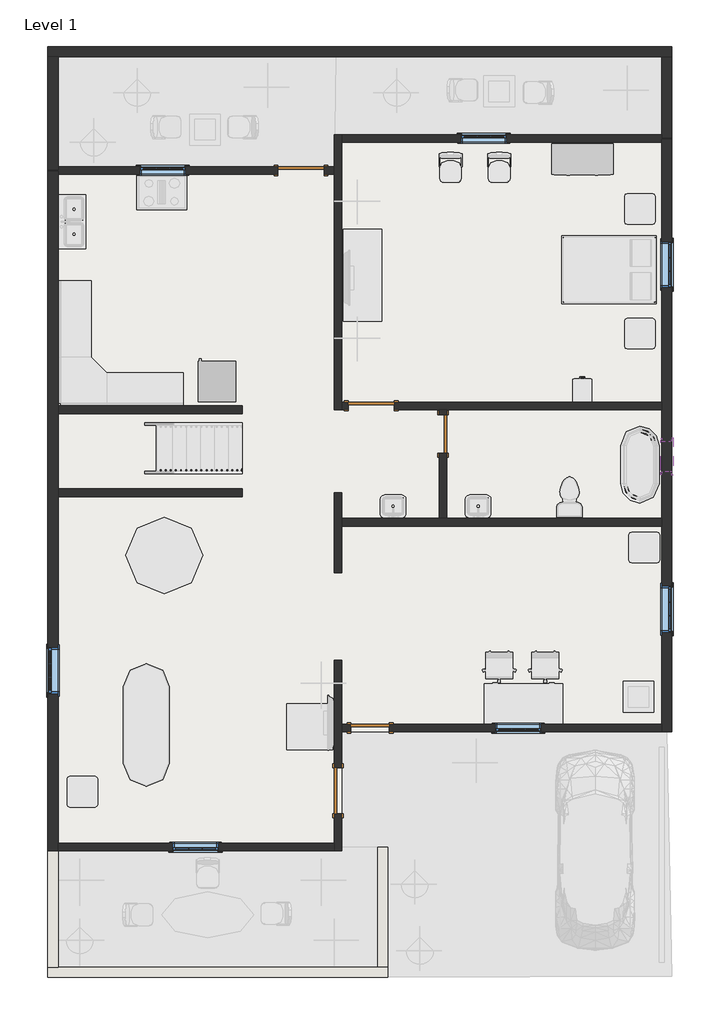
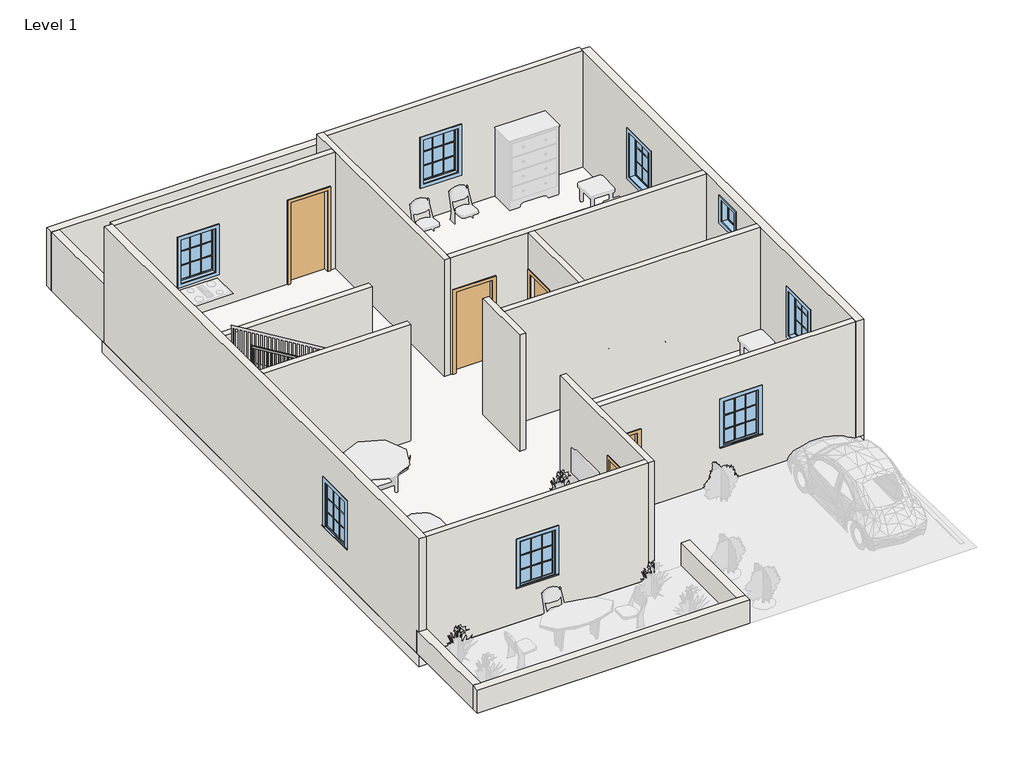
# One storey, part 1 of 2: 20 walls, 8 windows, 5 doors, 1 railing, 1 slab.
"""IFC4 building model written with IfcOpenShell, lengths in millimetres."""

from ifc_helpers import new_model, si_unit, frame, origin, origin_with_axes, place, context, project, spatial, polyline, outline, extrude, faceted_brep, transform, mapped, element, save
from components import door_255cab33, door_16372e1c, door_686f89d2, window_5c190c7e, window_29c06734, window_e41d21a6

model = new_model("IFC4")

# Units and contexts
model_context = context("Model", 3, world=origin())
ifc_project = project(units=[si_unit("LENGTHUNIT", "METRE", prefix="MILLI")], contexts=[model_context])

# Site, building, storey
site = spatial("IfcSite", under=ifc_project)
building = spatial("IfcBuilding", under=site)
storey = spatial("IfcBuildingStorey", under=building, Name="Level 1", Elevation=0.0)

# Doors
placement = place(None, origin())
door_shape = door_255cab33(model_context)
element("IfcDoor", 1, ObjectType="Single-Flush : 30\" x 80\"", at=placement, inside=storey, context=model_context, shape_type="MappedRepresentation", body=[
    mapped(door_shape, transform((1593.6745853, 5123.5742707, 0.0), x_axis=(0.0, 1.0, 0.0), y_axis=(-1.0, 0.0, 0.0), z_axis=(0.0, 0.0, 1.0))),
])
element("IfcDoor", 2, ObjectType="Single-Flush : 30\" x 80\"", at=placement, inside=storey, context=model_context, shape_type="MappedRepresentation", body=[
    mapped(door_shape, transform((145.8745853, -718.4257293, 0.0), x_axis=(-1.0, 0.0, 0.0), y_axis=(0.0, -1.0, 0.0), z_axis=(0.0, 0.0, 1.0))),
])
door_2_shape = door_16372e1c(model_context)
element("IfcDoor", 3, ObjectType="Single-Flush : 36\" x 84\"", at=placement, inside=storey, context=model_context, shape_type="MappedRepresentation", body=[
    mapped(door_2_shape, transform((-1225.7254147, 10355.9742707, 0.0), x_axis=(1.0, 0.0, 0.0), y_axis=(0.0, 1.0, 0.0), z_axis=(0.0, 0.0, 1.0))),
])
element("IfcDoor", 4, ObjectType="Single-Flush : 36\" x 84\"", at=placement, inside=storey, context=model_context, shape_type="MappedRepresentation", body=[
    mapped(door_2_shape, transform((-489.1254147, -1963.0257293, 0.0), x_axis=(0.0, 1.0, 0.0), y_axis=(-1.0, 0.0, 0.0), z_axis=(0.0, 0.0, 1.0))),
])
door_3_shape = door_686f89d2(model_context)
element("IfcDoor", 5, ObjectType="Single-Flush : 36\" x 84\"", at=placement, inside=storey, context=model_context, shape_type="MappedRepresentation", body=[
    mapped(door_3_shape, transform((171.2745853, 5682.3742707, 0.0), x_axis=(-1.0, 0.0, 0.0), y_axis=(0.0, -1.0, 0.0), z_axis=(0.0, 0.0, 1.0))),
])

# Railing
element("IfcRailing", 6, ObjectType="Handrail - Rectangular", at=placement, inside=storey, context=model_context, shape_type="SweptSolid", body=[
    extrude(outline(polyline([(1193.6652064, -2390.4214984), (1253.0666667, -2390.4214984), (3454.4, -6022.6214984), (3394.9985397, -6022.6214984), (1193.6652064, -2390.4214984)])), frame((0.0, 4382.4166905, 0.0), z_axis=(0.0, 1.0, 0.0), x_axis=(0.0, 0.0, 1.0)), (0.0, 0.0, 1.0), 50.8),
    extrude(outline(polyline([(3354.5894488, -5955.9464984), (2370.6666667, -5955.9464984), (2370.6666667, -5936.8964984), (3343.0439943, -5936.8964984), (3354.5894488, -5955.9464984)])), frame((0.0, 4398.2916905, 0.0), z_axis=(0.0, 1.0, 0.0), x_axis=(0.0, 0.0, 1.0)), (0.0, 0.0, 1.0), 19.05),
    extrude(outline(polyline([(3293.0136913, -5854.3464984), (2370.6666667, -5854.3464984), (2370.6666667, -5835.2964984), (3281.4682367, -5835.2964984), (3293.0136913, -5854.3464984)])), frame((0.0, 4398.2916905, 0.0), z_axis=(0.0, 1.0, 0.0), x_axis=(0.0, 0.0, 1.0)), (0.0, 0.0, 1.0), 19.05),
    extrude(outline(polyline([(3231.4379337, -5752.7464984), (2370.6666667, -5752.7464984), (2370.6666667, -5733.6964984), (3219.8924791, -5733.6964984), (3231.4379337, -5752.7464984)])), frame((0.0, 4398.2916905, 0.0), z_axis=(0.0, 1.0, 0.0), x_axis=(0.0, 0.0, 1.0)), (0.0, 0.0, 1.0), 19.05),
    extrude(outline(polyline([(3169.8621761, -5651.1464984), (2201.3333333, -5651.1464984), (2201.3333333, -5632.0964984), (3158.3167216, -5632.0964984), (3169.8621761, -5651.1464984)])), frame((0.0, 4398.2916905, 0.0), z_axis=(0.0, 1.0, 0.0), x_axis=(0.0, 0.0, 1.0)), (0.0, 0.0, 1.0), 19.05),
    extrude(outline(polyline([(3108.2864185, -5549.5464984), (2201.3333333, -5549.5464984), (2201.3333333, -5530.4964984), (3096.740964, -5530.4964984), (3108.2864185, -5549.5464984)])), frame((0.0, 4398.2916905, 0.0), z_axis=(0.0, 1.0, 0.0), x_axis=(0.0, 0.0, 1.0)), (0.0, 0.0, 1.0), 19.05),
    extrude(outline(polyline([(3046.710661, -5447.9464984), (2032.0, -5447.9464984), (2032.0, -5428.8964984), (3035.1652064, -5428.8964984), (3046.710661, -5447.9464984)])), frame((0.0, 4398.2916905, 0.0), z_axis=(0.0, 1.0, 0.0), x_axis=(0.0, 0.0, 1.0)), (0.0, 0.0, 1.0), 19.05),
    extrude(outline(polyline([(2985.1349034, -5346.3464984), (2032.0, -5346.3464984), (2032.0, -5327.2964984), (2973.5894488, -5327.2964984), (2985.1349034, -5346.3464984)])), frame((0.0, 4398.2916905, 0.0), z_axis=(0.0, 1.0, 0.0), x_axis=(0.0, 0.0, 1.0)), (0.0, 0.0, 1.0), 19.05),
    extrude(outline(polyline([(2923.5591458, -5244.7464984), (2032.0, -5244.7464984), (2032.0, -5225.6964984), (2912.0136913, -5225.6964984), (2923.5591458, -5244.7464984)])), frame((0.0, 4398.2916905, 0.0), z_axis=(0.0, 1.0, 0.0), x_axis=(0.0, 0.0, 1.0)), (0.0, 0.0, 1.0), 19.05),
    extrude(outline(polyline([(2861.9833882, -5143.1464984), (1862.6666667, -5143.1464984), (1862.6666667, -5124.0964984), (2850.4379337, -5124.0964984), (2861.9833882, -5143.1464984)])), frame((0.0, 4398.2916905, 0.0), z_axis=(0.0, 1.0, 0.0), x_axis=(0.0, 0.0, 1.0)), (0.0, 0.0, 1.0), 19.05),
    extrude(outline(polyline([(2800.4076307, -5041.5464984), (1862.6666667, -5041.5464984), (1862.6666667, -5022.4964984), (2788.8621761, -5022.4964984), (2800.4076307, -5041.5464984)])), frame((0.0, 4398.2916905, 0.0), z_axis=(0.0, 1.0, 0.0), x_axis=(0.0, 0.0, 1.0)), (0.0, 0.0, 1.0), 19.05),
    extrude(outline(polyline([(2738.8318731, -4939.9464984), (1862.6666667, -4939.9464984), (1862.6666667, -4920.8964984), (2727.2864185, -4920.8964984), (2738.8318731, -4939.9464984)])), frame((0.0, 4398.2916905, 0.0), z_axis=(0.0, 1.0, 0.0), x_axis=(0.0, 0.0, 1.0)), (0.0, 0.0, 1.0), 19.05),
    extrude(outline(polyline([(2677.2561155, -4838.3464984), (1693.3333333, -4838.3464984), (1693.3333333, -4819.2964984), (2665.710661, -4819.2964984), (2677.2561155, -4838.3464984)])), frame((0.0, 4398.2916905, 0.0), z_axis=(0.0, 1.0, 0.0), x_axis=(0.0, 0.0, 1.0)), (0.0, 0.0, 1.0), 19.05),
    extrude(outline(polyline([(2615.6803579, -4736.7464984), (1693.3333333, -4736.7464984), (1693.3333333, -4717.6964984), (2604.1349034, -4717.6964984), (2615.6803579, -4736.7464984)])), frame((0.0, 4398.2916905, 0.0), z_axis=(0.0, 1.0, 0.0), x_axis=(0.0, 0.0, 1.0)), (0.0, 0.0, 1.0), 19.05),
    extrude(outline(polyline([(2554.1046004, -4635.1464984), (1693.3333333, -4635.1464984), (1693.3333333, -4616.0964984), (2542.5591458, -4616.0964984), (2554.1046004, -4635.1464984)])), frame((0.0, 4398.2916905, 0.0), z_axis=(0.0, 1.0, 0.0), x_axis=(0.0, 0.0, 1.0)), (0.0, 0.0, 1.0), 19.05),
    extrude(outline(polyline([(2492.5288428, -4533.5464984), (1524.0, -4533.5464984), (1524.0, -4514.4964984), (2480.9833882, -4514.4964984), (2492.5288428, -4533.5464984)])), frame((0.0, 4398.2916905, 0.0), z_axis=(0.0, 1.0, 0.0), x_axis=(0.0, 0.0, 1.0)), (0.0, 0.0, 1.0), 19.05),
    extrude(outline(polyline([(2430.9530852, -4431.9464984), (1524.0, -4431.9464984), (1524.0, -4412.8964984), (2419.4076307, -4412.8964984), (2430.9530852, -4431.9464984)])), frame((0.0, 4398.2916905, 0.0), z_axis=(0.0, 1.0, 0.0), x_axis=(0.0, 0.0, 1.0)), (0.0, 0.0, 1.0), 19.05),
    extrude(outline(polyline([(2369.3773276, -4330.3464984), (1354.6666667, -4330.3464984), (1354.6666667, -4311.2964984), (2357.8318731, -4311.2964984), (2369.3773276, -4330.3464984)])), frame((0.0, 4398.2916905, 0.0), z_axis=(0.0, 1.0, 0.0), x_axis=(0.0, 0.0, 1.0)), (0.0, 0.0, 1.0), 19.05),
    extrude(outline(polyline([(2307.80157, -4228.7464984), (1354.6666667, -4228.7464984), (1354.6666667, -4209.6964984), (2296.2561155, -4209.6964984), (2307.80157, -4228.7464984)])), frame((0.0, 4398.2916905, 0.0), z_axis=(0.0, 1.0, 0.0), x_axis=(0.0, 0.0, 1.0)), (0.0, 0.0, 1.0), 19.05),
    extrude(outline(polyline([(2246.2258125, -4127.1464984), (1354.6666667, -4127.1464984), (1354.6666667, -4108.0964984), (2234.6803579, -4108.0964984), (2246.2258125, -4127.1464984)])), frame((0.0, 4398.2916905, 0.0), z_axis=(0.0, 1.0, 0.0), x_axis=(0.0, 0.0, 1.0)), (0.0, 0.0, 1.0), 19.05),
    extrude(outline(polyline([(2184.6500549, -4025.5464984), (1185.3333333, -4025.5464984), (1185.3333333, -4006.4964984), (2173.1046004, -4006.4964984), (2184.6500549, -4025.5464984)])), frame((0.0, 4398.2916905, 0.0), z_axis=(0.0, 1.0, 0.0), x_axis=(0.0, 0.0, 1.0)), (0.0, 0.0, 1.0), 19.05),
    extrude(outline(polyline([(2123.0742973, -3923.9464984), (1185.3333333, -3923.9464984), (1185.3333333, -3904.8964984), (2111.5288428, -3904.8964984), (2123.0742973, -3923.9464984)])), frame((0.0, 4398.2916905, 0.0), z_axis=(0.0, 1.0, 0.0), x_axis=(0.0, 0.0, 1.0)), (0.0, 0.0, 1.0), 19.05),
    extrude(outline(polyline([(2061.4985397, -3822.3464984), (1185.3333333, -3822.3464984), (1185.3333333, -3803.2964984), (2049.9530852, -3803.2964984), (2061.4985397, -3822.3464984)])), frame((0.0, 4398.2916905, 0.0), z_axis=(0.0, 1.0, 0.0), x_axis=(0.0, 0.0, 1.0)), (0.0, 0.0, 1.0), 19.05),
    extrude(outline(polyline([(1999.9227822, -3720.7464984), (1016.0, -3720.7464984), (1016.0, -3701.6964984), (1988.3773276, -3701.6964984), (1999.9227822, -3720.7464984)])), frame((0.0, 4398.2916905, 0.0), z_axis=(0.0, 1.0, 0.0), x_axis=(0.0, 0.0, 1.0)), (0.0, 0.0, 1.0), 19.05),
    extrude(outline(polyline([(1938.3470246, -3619.1464984), (1016.0, -3619.1464984), (1016.0, -3600.0964984), (1926.80157, -3600.0964984), (1938.3470246, -3619.1464984)])), frame((0.0, 4398.2916905, 0.0), z_axis=(0.0, 1.0, 0.0), x_axis=(0.0, 0.0, 1.0)), (0.0, 0.0, 1.0), 19.05),
    extrude(outline(polyline([(1876.771267, -3517.5464984), (1016.0, -3517.5464984), (1016.0, -3498.4964984), (1865.2258125, -3498.4964984), (1876.771267, -3517.5464984)])), frame((0.0, 4398.2916905, 0.0), z_axis=(0.0, 1.0, 0.0), x_axis=(0.0, 0.0, 1.0)), (0.0, 0.0, 1.0), 19.05),
    extrude(outline(polyline([(1815.1955094, -3415.9464984), (846.6666667, -3415.9464984), (846.6666667, -3396.8964984), (1803.6500549, -3396.8964984), (1815.1955094, -3415.9464984)])), frame((0.0, 4398.2916905, 0.0), z_axis=(0.0, 1.0, 0.0), x_axis=(0.0, 0.0, 1.0)), (0.0, 0.0, 1.0), 19.05),
    extrude(outline(polyline([(1753.6197519, -3314.3464984), (846.6666667, -3314.3464984), (846.6666667, -3295.2964984), (1742.0742973, -3295.2964984), (1753.6197519, -3314.3464984)])), frame((0.0, 4398.2916905, 0.0), z_axis=(0.0, 1.0, 0.0), x_axis=(0.0, 0.0, 1.0)), (0.0, 0.0, 1.0), 19.05),
    extrude(outline(polyline([(1692.0439943, -3212.7464984), (677.3333333, -3212.7464984), (677.3333333, -3193.6964984), (1680.4985397, -3193.6964984), (1692.0439943, -3212.7464984)])), frame((0.0, 4398.2916905, 0.0), z_axis=(0.0, 1.0, 0.0), x_axis=(0.0, 0.0, 1.0)), (0.0, 0.0, 1.0), 19.05),
    extrude(outline(polyline([(1630.4682367, -3111.1464984), (677.3333333, -3111.1464984), (677.3333333, -3092.0964984), (1618.9227822, -3092.0964984), (1630.4682367, -3111.1464984)])), frame((0.0, 4398.2916905, 0.0), z_axis=(0.0, 1.0, 0.0), x_axis=(0.0, 0.0, 1.0)), (0.0, 0.0, 1.0), 19.05),
    extrude(outline(polyline([(1568.8924791, -3009.5464984), (677.3333333, -3009.5464984), (677.3333333, -2990.4964984), (1557.3470246, -2990.4964984), (1568.8924791, -3009.5464984)])), frame((0.0, 4398.2916905, 0.0), z_axis=(0.0, 1.0, 0.0), x_axis=(0.0, 0.0, 1.0)), (0.0, 0.0, 1.0), 19.05),
    extrude(outline(polyline([(1507.3167216, -2907.9464984), (508.0, -2907.9464984), (508.0, -2888.8964984), (1495.771267, -2888.8964984), (1507.3167216, -2907.9464984)])), frame((0.0, 4398.2916905, 0.0), z_axis=(0.0, 1.0, 0.0), x_axis=(0.0, 0.0, 1.0)), (0.0, 0.0, 1.0), 19.05),
    extrude(outline(polyline([(1445.740964, -2806.3464984), (508.0, -2806.3464984), (508.0, -2787.2964984), (1434.1955094, -2787.2964984), (1445.740964, -2806.3464984)])), frame((0.0, 4398.2916905, 0.0), z_axis=(0.0, 1.0, 0.0), x_axis=(0.0, 0.0, 1.0)), (0.0, 0.0, 1.0), 19.05),
    extrude(outline(polyline([(1384.1652064, -2704.7464984), (508.0, -2704.7464984), (508.0, -2685.6964984), (1372.6197519, -2685.6964984), (1384.1652064, -2704.7464984)])), frame((0.0, 4398.2916905, 0.0), z_axis=(0.0, 1.0, 0.0), x_axis=(0.0, 0.0, 1.0)), (0.0, 0.0, 1.0), 19.05),
    extrude(outline(polyline([(1322.5894488, -2603.1464984), (338.6666667, -2603.1464984), (338.6666667, -2584.0964984), (1311.0439943, -2584.0964984), (1322.5894488, -2603.1464984)])), frame((0.0, 4398.2916905, 0.0), z_axis=(0.0, 1.0, 0.0), x_axis=(0.0, 0.0, 1.0)), (0.0, 0.0, 1.0), 19.05),
    extrude(outline(polyline([(1261.0136913, -2501.5464984), (338.6666667, -2501.5464984), (338.6666667, -2482.4964984), (1249.4682367, -2482.4964984), (1261.0136913, -2501.5464984)])), frame((0.0, 4398.2916905, 0.0), z_axis=(0.0, 1.0, 0.0), x_axis=(0.0, 0.0, 1.0)), (0.0, 0.0, 1.0), 19.05),
    extrude(outline(polyline([(3394.9985397, -6022.6214984), (2370.6666667, -6022.6214984), (2370.6666667, -6003.5714984), (3383.4530852, -6003.5714984), (3394.9985397, -6022.6214984)])), frame((0.0, 4398.2916905, 0.0), z_axis=(0.0, 1.0, 0.0), x_axis=(0.0, 0.0, 1.0)), (0.0, 0.0, 1.0), 19.05),
    extrude(outline(polyline([(1205.210661, -2409.4714984), (338.6666667, -2409.4714984), (338.6666667, -2390.4214984), (1193.6652064, -2390.4214984), (1205.210661, -2409.4714984)])), frame((0.0, 4398.2916905, 0.0), z_axis=(0.0, 1.0, 0.0), x_axis=(0.0, 0.0, 1.0)), (0.0, 0.0, 1.0), 19.05),
])

# Slab
element("IfcSlab", 7, ObjectType="Generic - 12\"", at=placement, inside=storey, context=model_context, shape_type="SweptSolid", body=[
    extrude(outline(polyline([(-565.3254147, 10432.1742707), (-565.3254147, 11067.1742707), (6140.2745853, 11067.1742707), (6140.2745853, -794.6257293), (-412.9254147, -794.6257293), (-412.9254147, -3156.8257293), (-6254.9254147, -3156.8257293), (-6254.9254147, 10432.1742707), (-565.3254147, 10432.1742707)])), frame((0.0, 0.0, -304.8), z_axis=(0.0, 0.0, 1.0), x_axis=(1.0, 0.0, 0.0)), (0.0, 0.0, 1.0), 304.8),
])

# Walls
element("IfcWall", 8, ObjectType="Generic - 8\"", at=placement, inside=storey, context=model_context, shape_type="Brep", body=[
    faceted_brep([(-6051.7254147, -3080.6257293, 0.0), (-6051.7254147, -3004.4257293, 0.0), (-6051.7254147, 3878.9742707, 0.0), (-6051.7254147, 4031.3742707, 0.0), (-6051.7254147, 5529.9742707, 0.0), (-6051.7254147, 5682.3742707, 0.0), (-6051.7254147, 10343.2742707, 0.0), (-6051.7254147, 10343.2742707, 3048.0), (-6051.7254147, 5682.3742707, 3048.0), (-6051.7254147, 5529.9742707, 3048.0), (-6051.7254147, 4031.3742707, 3048.0), (-6051.7254147, 3878.9742707, 3048.0), (-6051.7254147, -3004.4257293, 3048.0), (-6051.7254147, -3156.8257293, 3048.0), (-6051.7254147, -3156.8257293, 609.6), (-6051.7254147, -3080.6257293, 609.6), (-6051.7254147, 881.7742707, 2133.6), (-6051.7254147, 881.7742707, 914.4), (-6051.7254147, -32.6257293, 914.4), (-6051.7254147, -32.6257293, 2133.6), (-6254.9254147, -3080.6257293, 0.0), (-6254.9254147, -3080.6257293, 609.6), (-6254.9254147, -3156.8257293, 609.6), (-6254.9254147, -3156.8257293, 3048.0), (-6254.9254147, 10343.2742707, 3048.0), (-6254.9254147, 10343.2742707, 0.0), (-6254.9254147, 881.7742707, 2133.6), (-6254.9254147, -32.6257293, 2133.6), (-6254.9254147, -32.6257293, 914.4), (-6254.9254147, 881.7742707, 914.4)], [[[0, 1, 2, 3, 4, 5, 6, 7, 8, 9, 10, 11, 12, 13, 14, 15], [16, 17, 18, 19]], [[20, 21, 22, 23, 24, 25], [26, 27, 28, 29]], [[6, 5, 4, 3, 2, 1, 0, 20, 25]], [[7, 6, 25, 24]], [[0, 15, 21, 20]], [[14, 22, 21, 15]], [[14, 13, 23, 22]], [[17, 16, 26, 29]], [[18, 17, 29, 28]], [[19, 18, 28, 27]], [[16, 19, 27, 26]], [[13, 12, 11, 10, 9, 8, 7, 24, 23]]]),
])
element("IfcWall", 9, ObjectType="Generic - 8\"", at=placement, inside=storey, context=model_context, shape_type="Brep", body=[
    faceted_brep([(5937.0745853, 10978.2742707, 0.0), (5937.0745853, 10914.7742707, 0.0), (5937.0745853, 5758.5742707, 0.0), (5937.0745853, 5606.1742707, 0.0), (5937.0745853, 3447.1742707, 0.0), (5937.0745853, 3294.7742707, 0.0), (5937.0745853, -642.2257293, 0.0), (5937.0745853, -794.6257293, 0.0), (5937.0745853, -794.6257293, 3048.0), (5937.0745853, -642.2257293, 3048.0), (5937.0745853, 3294.7742707, 3048.0), (5937.0745853, 3447.1742707, 3048.0), (5937.0745853, 5606.1742707, 3048.0), (5937.0745853, 5758.5742707, 3048.0), (5937.0745853, 10914.7742707, 3048.0), (5937.0745853, 10978.2742707, 3048.0), (5937.0745853, 8031.8742707, 2133.6), (5937.0745853, 8031.8742707, 914.4), (5937.0745853, 8946.2742707, 914.4), (5937.0745853, 8946.2742707, 2133.6), (5937.0745853, 1186.5742707, 2133.6), (5937.0745853, 1186.5742707, 914.4), (5937.0745853, 2100.9742707, 914.4), (5937.0745853, 2100.9742707, 2133.6), (5937.0745853, 4374.2742707, 2768.6), (5937.0745853, 4374.2742707, 2159.0), (5937.0745853, 4983.8742707, 2159.0), (5937.0745853, 4983.8742707, 2768.6), (6140.2745853, 10978.2742707, 0.0), (6140.2745853, 10978.2742707, 3048.0), (6140.2745853, -794.6257293, 3048.0), (6140.2745853, -794.6257293, 0.0), (6140.2745853, 8031.8742707, 2133.6), (6140.2745853, 8946.2742707, 2133.6), (6140.2745853, 8946.2742707, 914.4), (6140.2745853, 8031.8742707, 914.4), (6140.2745853, 1186.5742707, 2133.6), (6140.2745853, 2100.9742707, 2133.6), (6140.2745853, 2100.9742707, 914.4), (6140.2745853, 1186.5742707, 914.4), (6140.2745853, 4374.2742707, 2768.6), (6140.2745853, 4983.8742707, 2768.6), (6140.2745853, 4983.8742707, 2159.0), (6140.2745853, 4374.2742707, 2159.0)], [[[0, 1, 2, 3, 4, 5, 6, 7, 8, 9, 10, 11, 12, 13, 14, 15], [16, 17, 18, 19], [20, 21, 22, 23], [24, 25, 26, 27]], [[28, 29, 30, 31], [32, 33, 34, 35], [36, 37, 38, 39], [40, 41, 42, 43]], [[7, 6, 5, 4, 3, 2, 1, 0, 28, 31]], [[0, 15, 29, 28]], [[8, 7, 31, 30]], [[16, 19, 33, 32]], [[19, 18, 34, 33]], [[18, 17, 35, 34]], [[17, 16, 32, 35]], [[20, 23, 37, 36]], [[23, 22, 38, 37]], [[22, 21, 39, 38]], [[21, 20, 36, 39]], [[24, 27, 41, 40]], [[27, 26, 42, 41]], [[26, 25, 43, 42]], [[25, 24, 40, 43]], [[15, 14, 13, 12, 11, 10, 9, 8, 30, 29]]]),
])
element("IfcWall", 10, ObjectType="Generic - 8\" 2", at=placement, inside=storey, context=model_context, shape_type="Brep", body=[
    faceted_brep([(-6254.9254147, 12616.5742707, 0.0), (-6051.7254147, 12616.5742707, 0.0), (5937.0745853, 12616.5742707, 0.0), (6140.2745853, 12616.5742707, 0.0), (6140.2745853, 12616.5742707, 1524.0), (5937.0745853, 12616.5742707, 1524.0), (-6051.7254147, 12616.5742707, 1524.0), (-6254.9254147, 12616.5742707, 1524.0), (-6254.9254147, 12819.7742707, 0.0), (-6254.9254147, 12819.7742707, 1524.0), (6140.2745853, 12819.7742707, 1524.0), (6140.2745853, 12819.7742707, 0.0)], [[[0, 1, 2, 3, 4, 5, 6, 7]], [[8, 9, 10, 11]], [[3, 2, 1, 0, 8, 11]], [[7, 6, 5, 4, 10, 9]], [[4, 3, 11, 10]], [[0, 7, 9, 8]]]),
])
element("IfcWall", 11, ObjectType="Generic - 8\" 2", at=placement, inside=storey, context=model_context, shape_type="SweptSolid", body=[
    extrude(outline(polyline([(5937.0745853, 11003.6742707), (5937.0745853, 12616.5742707), (6140.2745853, 12616.5742707), (6140.2745853, 11003.6742707), (5937.0745853, 11003.6742707)])), origin_with_axes(), (0.0, 0.0, 1.0), 1524.0),
])
element("IfcWall", 12, ObjectType="Generic - 8\" 2", at=placement, inside=storey, context=model_context, shape_type="Brep", body=[
    faceted_brep([(-6051.7254147, -5468.2257293, 0.0), (-6051.7254147, -3156.8257293, 0.0), (-6051.7254147, -3080.6257293, 0.0), (-6051.7254147, -3080.6257293, 609.6), (-6051.7254147, -5468.2257293, 609.6), (-6254.9254147, -5468.2257293, 0.0), (-6254.9254147, -5468.2257293, 609.6), (-6254.9254147, -3080.6257293, 609.6), (-6254.9254147, -3080.6257293, 0.0)], [[[0, 1, 2, 3, 4]], [[5, 6, 7, 8]], [[2, 1, 0, 5, 8]], [[3, 2, 8, 7]], [[4, 3, 7, 6]], [[0, 4, 6, 5]]]),
])
element("IfcWall", 13, ObjectType="Generic - 8\" 2", at=placement, inside=storey, context=model_context, shape_type="Brep", body=[
    faceted_brep([(501.4745853, -5468.2257293, 0.0), (298.2745853, -5468.2257293, 0.0), (-6051.7254147, -5468.2257293, 0.0), (-6254.9254147, -5468.2257293, 0.0), (-6254.9254147, -5468.2257293, 609.6), (-6051.7254147, -5468.2257293, 609.6), (298.2745853, -5468.2257293, 609.6), (501.4745853, -5468.2257293, 609.6), (501.4745853, -5671.4257293, 0.0), (501.4745853, -5671.4257293, 609.6), (-6254.9254147, -5671.4257293, 609.6), (-6254.9254147, -5671.4257293, 0.0)], [[[0, 1, 2, 3, 4, 5, 6, 7]], [[8, 9, 10, 11]], [[3, 2, 1, 0, 8, 11]], [[7, 6, 5, 4, 10, 9]], [[4, 3, 11, 10]], [[0, 7, 9, 8]]]),
])
element("IfcWall", 14, ObjectType="Generic - 8\" 2", at=placement, inside=storey, context=model_context, shape_type="SweptSolid", body=[
    extrude(outline(polyline([(298.2745853, -5468.2257293), (298.2745853, -3080.6257293), (501.4745853, -3080.6257293), (501.4745853, -5468.2257293), (298.2745853, -5468.2257293)])), origin_with_axes(), (0.0, 0.0, 1.0), 609.6),
])
element("IfcWall", 15, ObjectType="Generic - 8\" 2", at=placement, inside=storey, context=model_context, shape_type="Brep", body=[
    faceted_brep([(-6051.7254147, 10368.6742707, 0.0), (-6051.7254147, 10432.1742707, 0.0), (-6051.7254147, 12616.5742707, 0.0), (-6051.7254147, 12616.5742707, 1524.0), (-6051.7254147, 10368.6742707, 1524.0), (-6254.9254147, 10368.6742707, 0.0), (-6254.9254147, 10368.6742707, 1524.0), (-6254.9254147, 12616.5742707, 1524.0), (-6254.9254147, 12616.5742707, 0.0)], [[[0, 1, 2, 3, 4]], [[5, 6, 7, 8]], [[2, 1, 0, 5, 8]], [[4, 3, 7, 6]], [[0, 4, 6, 5]], [[3, 2, 8, 7]]]),
])
element("IfcWall", 16, ObjectType="INNER WALL 6\"", at=placement, inside=storey, context=model_context, shape_type="Brep", body=[
    faceted_brep([(-768.5254147, 10279.7742707, 2133.6), (-768.5254147, 10279.7742707, 0.0), (-565.3254147, 10279.7742707, 0.0), (-565.3254147, 10279.7742707, 3048.0), (-6051.7254147, 10279.7742707, 3048.0), (-6051.7254147, 10279.7742707, 0.0), (-1682.9254147, 10279.7742707, 0.0), (-1682.9254147, 10279.7742707, 2133.6), (-3511.7254147, 10279.7742707, 2133.6), (-3511.7254147, 10279.7742707, 914.4), (-4426.1254147, 10279.7742707, 914.4), (-4426.1254147, 10279.7742707, 2133.6), (-565.3254147, 10432.1742707, 0.0), (-768.5254147, 10432.1742707, 0.0), (-768.5254147, 10432.1742707, 2133.6), (-1682.9254147, 10432.1742707, 2133.6), (-1682.9254147, 10432.1742707, 0.0), (-6051.7254147, 10432.1742707, 0.0), (-6051.7254147, 10432.1742707, 3048.0), (-565.3254147, 10432.1742707, 3048.0), (-3511.7254147, 10432.1742707, 2133.6), (-4426.1254147, 10432.1742707, 2133.6), (-4426.1254147, 10432.1742707, 914.4), (-3511.7254147, 10432.1742707, 914.4), (-6051.7254147, 10368.6742707, 0.0)], [[[0, 1, 2, 3, 4, 5, 6, 7], [8, 9, 10, 11]], [[12, 13, 14, 15, 16, 17, 18, 19], [20, 21, 22, 23]], [[6, 5, 24, 17, 16]], [[2, 1, 13, 12]], [[5, 4, 18, 17, 24]], [[3, 2, 12, 19]], [[14, 13, 1, 0]], [[15, 14, 0, 7]], [[16, 15, 7, 6]], [[9, 8, 20, 23]], [[10, 9, 23, 22]], [[11, 10, 22, 21]], [[8, 11, 21, 20]], [[4, 3, 19, 18]]]),
])
element("IfcWall", 17, ObjectType="INNER WALL 6\"", at=placement, inside=storey, context=model_context, shape_type="Brep", body=[
    faceted_brep([(-412.9254147, 5606.1742707, 0.0), (-412.9254147, 5758.5742707, 0.0), (-412.9254147, 10914.7742707, 0.0), (-412.9254147, 11067.1742707, 0.0), (-412.9254147, 11067.1742707, 3048.0), (-412.9254147, 10914.7742707, 3048.0), (-412.9254147, 5758.5742707, 3048.0), (-412.9254147, 5606.1742707, 3048.0), (-565.3254147, 5606.1742707, 0.0), (-565.3254147, 5606.1742707, 3048.0), (-565.3254147, 10279.7742707, 3048.0), (-565.3254147, 10432.1742707, 3048.0), (-565.3254147, 11067.1742707, 3048.0), (-565.3254147, 11067.1742707, 0.0), (-565.3254147, 10432.1742707, 0.0), (-565.3254147, 10279.7742707, 0.0)], [[[0, 1, 2, 3, 4, 5, 6, 7]], [[8, 9, 10, 11, 12, 13, 14, 15]], [[3, 2, 1, 0, 8, 15, 14, 13]], [[4, 3, 13, 12]], [[0, 7, 9, 8]], [[7, 6, 5, 4, 12, 11, 10, 9]]]),
])
element("IfcWall", 18, ObjectType="INNER WALL 6\"", at=placement, inside=storey, context=model_context, shape_type="Brep", body=[
    faceted_brep([(-412.9254147, 10914.7742707, 0.0), (5937.0745853, 10914.7742707, 0.0), (5937.0745853, 10914.7742707, 3048.0), (-412.9254147, 10914.7742707, 3048.0), (2863.6745853, 10914.7742707, 2133.6), (2863.6745853, 10914.7742707, 914.4), (1949.2745853, 10914.7742707, 914.4), (1949.2745853, 10914.7742707, 2133.6), (-412.9254147, 11067.1742707, 0.0), (-412.9254147, 11067.1742707, 3048.0), (5937.0745853, 11067.1742707, 3048.0), (5937.0745853, 11067.1742707, 0.0), (2863.6745853, 11067.1742707, 2133.6), (1949.2745853, 11067.1742707, 2133.6), (1949.2745853, 11067.1742707, 914.4), (2863.6745853, 11067.1742707, 914.4), (5937.0745853, 10978.2742707, 0.0), (5937.0745853, 10978.2742707, 3048.0)], [[[0, 1, 2, 3], [4, 5, 6, 7]], [[8, 9, 10, 11], [12, 13, 14, 15]], [[1, 0, 8, 11, 16]], [[0, 3, 9, 8]], [[2, 1, 16, 11, 10, 17]], [[5, 4, 12, 15]], [[6, 5, 15, 14]], [[7, 6, 14, 13]], [[4, 7, 13, 12]], [[3, 2, 17, 10, 9]]]),
])
element("IfcWall", 19, ObjectType="INNER WALL 6\"", at=placement, inside=storey, context=model_context, shape_type="Brep", body=[
    faceted_brep([(-285.9254147, 5758.5742707, 2133.6), (-285.9254147, 5758.5742707, 0.0), (-412.9254147, 5758.5742707, 0.0), (-412.9254147, 5758.5742707, 3048.0), (5937.0745853, 5758.5742707, 3048.0), (5937.0745853, 5758.5742707, 0.0), (628.4745853, 5758.5742707, 0.0), (628.4745853, 5758.5742707, 2133.6), (-412.9254147, 5606.1742707, 0.0), (-285.9254147, 5606.1742707, 0.0), (-285.9254147, 5606.1742707, 2133.6), (628.4745853, 5606.1742707, 2133.6), (628.4745853, 5606.1742707, 0.0), (1517.4745853, 5606.1742707, 0.0), (1669.8745853, 5606.1742707, 0.0), (5937.0745853, 5606.1742707, 0.0), (5937.0745853, 5606.1742707, 3048.0), (1669.8745853, 5606.1742707, 3048.0), (1517.4745853, 5606.1742707, 3048.0), (-412.9254147, 5606.1742707, 3048.0)], [[[0, 1, 2, 3, 4, 5, 6, 7]], [[8, 9, 10, 11, 12, 13, 14, 15, 16, 17, 18, 19]], [[6, 5, 15, 14, 13, 12]], [[2, 1, 9, 8]], [[5, 4, 16, 15]], [[10, 9, 1, 0]], [[11, 10, 0, 7]], [[12, 11, 7, 6]], [[3, 2, 8, 19]], [[4, 3, 19, 18, 17, 16]]]),
])
element("IfcWall", 20, ObjectType="INNER WALL 6\"", at=placement, inside=storey, context=model_context, shape_type="SweptSolid", body=[
    extrude(outline(polyline([(-6051.7254147, 5682.3742707), (-2394.1254147, 5682.3742707), (-2394.1254147, 5529.9742707), (-6051.7254147, 5529.9742707), (-6051.7254147, 5682.3742707)])), origin_with_axes(), (0.0, 0.0, 1.0), 3048.0),
])
element("IfcWall", 21, ObjectType="INNER WALL 6\"", at=placement, inside=storey, context=model_context, shape_type="SweptSolid", body=[
    extrude(outline(polyline([(-6051.7254147, 4031.3742707), (-2394.1254147, 4031.3742707), (-2394.1254147, 3878.9742707), (-6051.7254147, 3878.9742707), (-6051.7254147, 4031.3742707)])), origin_with_axes(), (0.0, 0.0, 1.0), 3048.0),
])
element("IfcWall", 22, ObjectType="INNER WALL 6\"", at=placement, inside=storey, context=model_context, shape_type="Brep", body=[
    faceted_brep([(-565.3254147, 3955.1742707, 0.0), (-565.3254147, 2367.6742707, 0.0), (-565.3254147, 2367.6742707, 3048.0), (-565.3254147, 3955.1742707, 3048.0), (-412.9254147, 3955.1742707, 0.0), (-412.9254147, 3955.1742707, 3048.0), (-412.9254147, 3447.1742707, 3048.0), (-412.9254147, 3294.7742707, 3048.0), (-412.9254147, 2367.6742707, 3048.0), (-412.9254147, 2367.6742707, 0.0), (-412.9254147, 3294.7742707, 0.0), (-412.9254147, 3447.1742707, 0.0)], [[[0, 1, 2, 3]], [[4, 5, 6, 7, 8, 9, 10, 11]], [[1, 0, 4, 11, 10, 9]], [[2, 1, 9, 8]], [[0, 3, 5, 4]], [[3, 2, 8, 7, 6, 5]]]),
])
element("IfcWall", 23, ObjectType="INNER WALL 6\"", at=placement, inside=storey, context=model_context, shape_type="Brep", body=[
    faceted_brep([(-412.9254147, 3294.7742707, 0.0), (5937.0745853, 3294.7742707, 0.0), (5937.0745853, 3294.7742707, 3048.0), (-412.9254147, 3294.7742707, 3048.0), (-412.9254147, 3447.1742707, 0.0), (-412.9254147, 3447.1742707, 3048.0), (1517.4745853, 3447.1742707, 3048.0), (1669.8745853, 3447.1742707, 3048.0), (5937.0745853, 3447.1742707, 3048.0), (5937.0745853, 3447.1742707, 0.0), (1669.8745853, 3447.1742707, 0.0), (1517.4745853, 3447.1742707, 0.0)], [[[0, 1, 2, 3]], [[4, 5, 6, 7, 8, 9, 10, 11]], [[1, 0, 4, 11, 10, 9]], [[2, 1, 9, 8]], [[0, 3, 5, 4]], [[3, 2, 8, 7, 6, 5]]]),
])
element("IfcWall", 24, ObjectType="INNER WALL 6\"", at=placement, inside=storey, context=model_context, shape_type="SweptSolid", body=[
    extrude(outline(polyline([(5606.1742707, 3048.0), (5606.1742707, 0.0), (5504.5742707, 0.0), (5504.5742707, 2032.0), (4742.5742707, 2032.0), (4742.5742707, 0.0), (3447.1742707, 0.0), (3447.1742707, 3048.0), (5606.1742707, 3048.0)])), frame((1517.4745853, 0.0, 0.0), z_axis=(1.0, 0.0, 0.0), x_axis=(0.0, 1.0, 0.0)), (0.0, 0.0, 1.0), 152.4),
])
element("IfcWall", 25, ObjectType="INNER WALL 6\"", at=placement, inside=storey, context=model_context, shape_type="SweptSolid", body=[
    extrude(outline(polyline([(0.0, -412.9254147), (0.0, -235.1254147), (2032.0, -235.1254147), (2032.0, 526.8745853), (0.0, 526.8745853), (0.0, 5937.0745853), (3048.0, 5937.0745853), (3048.0, -412.9254147), (0.0, -412.9254147)]), holes=[polyline([(2133.6, 2635.0745853), (2133.6, 3549.4745853), (914.4, 3549.4745853), (914.4, 2635.0745853), (2133.6, 2635.0745853)])]), frame((0.0, -794.6257293, 0.0), z_axis=(0.0, 1.0, 0.0), x_axis=(0.0, 0.0, 1.0)), (0.0, 0.0, 1.0), 152.4),
])
element("IfcWall", 26, ObjectType="INNER WALL 6\"", at=placement, inside=storey, context=model_context, shape_type="Brep", body=[
    faceted_brep([(-565.3254147, -3004.4257293, 0.0), (-6051.7254147, -3004.4257293, 0.0), (-6051.7254147, -3004.4257293, 3048.0), (-565.3254147, -3004.4257293, 3048.0), (-3778.4254147, -3004.4257293, 2133.6), (-3778.4254147, -3004.4257293, 914.4), (-2864.0254147, -3004.4257293, 914.4), (-2864.0254147, -3004.4257293, 2133.6), (-565.3254147, -3156.8257293, 0.0), (-565.3254147, -3156.8257293, 3048.0), (-6051.7254147, -3156.8257293, 3048.0), (-6051.7254147, -3156.8257293, 609.6), (-6051.7254147, -3156.8257293, 0.0), (-3778.4254147, -3156.8257293, 2133.6), (-2864.0254147, -3156.8257293, 2133.6), (-2864.0254147, -3156.8257293, 914.4), (-3778.4254147, -3156.8257293, 914.4), (-6051.7254147, -3080.6257293, 0.0)], [[[0, 1, 2, 3], [4, 5, 6, 7]], [[8, 9, 10, 11, 12], [13, 14, 15, 16]], [[1, 0, 8, 12, 17]], [[0, 3, 9, 8]], [[1, 17, 12, 11, 10, 2]], [[5, 4, 13, 16]], [[6, 5, 16, 15]], [[7, 6, 15, 14]], [[4, 7, 14, 13]], [[3, 2, 10, 9]]]),
])
element("IfcWall", 27, ObjectType="INNER WALL 6\"", at=placement, inside=storey, context=model_context, shape_type="Brep", body=[
    faceted_brep([(-565.3254147, 627.7742707, 0.0), (-565.3254147, -1505.8257293, 0.0), (-565.3254147, -1505.8257293, 2133.6), (-565.3254147, -2420.2257293, 2133.6), (-565.3254147, -2420.2257293, 0.0), (-565.3254147, -3004.4257293, 0.0), (-565.3254147, -3156.8257293, 0.0), (-565.3254147, -3156.8257293, 3048.0), (-565.3254147, -3004.4257293, 3048.0), (-565.3254147, 627.7742707, 3048.0), (-412.9254147, -1505.8257293, 2133.6), (-412.9254147, -1505.8257293, 0.0), (-412.9254147, -794.6257293, 0.0), (-412.9254147, -642.2257293, 0.0), (-412.9254147, 627.7742707, 0.0), (-412.9254147, 627.7742707, 3048.0), (-412.9254147, -642.2257293, 3048.0), (-412.9254147, -794.6257293, 3048.0), (-412.9254147, -3156.8257293, 3048.0), (-412.9254147, -3156.8257293, 0.0), (-412.9254147, -2420.2257293, 0.0), (-412.9254147, -2420.2257293, 2133.6)], [[[0, 1, 2, 3, 4, 5, 6, 7, 8, 9]], [[10, 11, 12, 13, 14, 15, 16, 17, 18, 19, 20, 21]], [[20, 19, 6, 5, 4]], [[14, 13, 12, 11, 1, 0]], [[0, 9, 15, 14]], [[7, 6, 19, 18]], [[4, 3, 21, 20]], [[3, 2, 10, 21]], [[2, 1, 11, 10]], [[9, 8, 7, 18, 17, 16, 15]]]),
])

# Windows
window_shape = window_5c190c7e(model_context)
element("IfcWindow", 28, ObjectType="Casement 3x3 with Trim : 36\" x 48\"", at=placement, inside=storey, context=model_context, shape_type="MappedRepresentation", body=[
    mapped(window_shape, transform((-3968.9254147, 10355.9742707, 0.0), x_axis=(1.0, 0.0, 0.0), y_axis=(0.0, 1.0, 0.0), z_axis=(0.0, 0.0, 1.0))),
])
element("IfcWindow", 29, ObjectType="Casement 3x3 with Trim : 36\" x 48\"", at=placement, inside=storey, context=model_context, shape_type="MappedRepresentation", body=[
    mapped(window_shape, transform((2406.4745853, 10990.9742707, 0.0), x_axis=(1.0, 0.0, 0.0), y_axis=(0.0, 1.0, 0.0), z_axis=(0.0, 0.0, 1.0))),
])
element("IfcWindow", 30, ObjectType="Casement 3x3 with Trim : 36\" x 48\"", at=placement, inside=storey, context=model_context, shape_type="MappedRepresentation", body=[
    mapped(window_shape, transform((3092.2745853, -718.4257293, 0.0), x_axis=(-1.0, 0.0, 0.0), y_axis=(0.0, -1.0, 0.0), z_axis=(0.0, 0.0, 1.0))),
])
element("IfcWindow", 31, ObjectType="Casement 3x3 with Trim : 36\" x 48\"", at=placement, inside=storey, context=model_context, shape_type="MappedRepresentation", body=[
    mapped(window_shape, transform((-3321.2254147, -3080.6257293, 0.0), x_axis=(-1.0, 0.0, 0.0), y_axis=(0.0, -1.0, 0.0), z_axis=(0.0, 0.0, 1.0))),
])
window_2_shape = window_29c06734(model_context)
element("IfcWindow", 32, ObjectType="Casement 3x3 with Trim : 36\" x 48\"", at=placement, inside=storey, context=model_context, shape_type="MappedRepresentation", body=[
    mapped(window_2_shape, transform((6038.6745853, 8489.0742707, 0.0), x_axis=(0.0, -1.0, 0.0), y_axis=(1.0, 0.0, 0.0), z_axis=(0.0, 0.0, 1.0))),
])
element("IfcWindow", 33, ObjectType="Casement 3x3 with Trim : 36\" x 48\"", at=placement, inside=storey, context=model_context, shape_type="MappedRepresentation", body=[
    mapped(window_2_shape, transform((6038.6745853, 1643.7742707, 0.0), x_axis=(0.0, -1.0, 0.0), y_axis=(1.0, 0.0, 0.0), z_axis=(0.0, 0.0, 1.0))),
])
element("IfcWindow", 34, ObjectType="Casement 3x3 with Trim : 36\" x 48\"", at=placement, inside=storey, context=model_context, shape_type="MappedRepresentation", body=[
    mapped(window_2_shape, transform((-6153.3254147, 424.5742707, 0.0), x_axis=(0.0, 1.0, 0.0), y_axis=(-1.0, 0.0, 0.0), z_axis=(0.0, 0.0, 1.0))),
])
window_3_shape = window_e41d21a6(model_context)
element("IfcWindow", 35, ObjectType="Transom with Trim : 24\" x 24\"", at=placement, inside=storey, context=model_context, shape_type="MappedRepresentation", body=[
    mapped(window_3_shape, transform((6038.6745853, 4640.9742707, 0.0), x_axis=(0.0, -1.0, 0.0), y_axis=(1.0, 0.0, 0.0), z_axis=(0.0, 0.0, 1.0))),
])

save(model, "model.ifc")

# Revit data of these elements
# Type "Single-Flush : 30\" x 80\""
#   Type Mark = "5"
#   Construction Type Id = "MDOOR"
#   Assembly Code = "C1020"
#   Analytic Construction = "Metal"
#   Thickness = 0' - 2"
#   Heat Transfer Coefficient (U) = 0.651978 BTU/(h·ft²·°F)
#   Height = 6' - 8"
#   Trim Projection Ext = 0' - 1"
#   Trim Projection Int = 0' - 1"
#   Trim Width = 0' - 3"
#   Width = 2' - 6"
#   Define Thermal Properties by = 1
#   Door Material = Door - Panel
#   Frame Material = Door - Frame
#   Visual Light Transmittance = 0
#   Solar Heat Gain Coefficient = 0
#   Function = (empty or 0)
#   Wall Closure = (empty or 0)
# Type "Single-Flush : 36\" x 84\""
#   Type Mark = "1"
#   Construction Type Id = "MDOOR"
#   Assembly Code = "C1020"
#   Analytic Construction = "Metal"
#   Thickness = 0' - 2"
#   Heat Transfer Coefficient (U) = 0.651978 BTU/(h·ft²·°F)
#   Height = 7' - 0"
#   Trim Projection Ext = 0' - 1"
#   Trim Projection Int = 0' - 1"
#   Trim Width = 0' - 3"
#   Width = 3' - 0"
#   Define Thermal Properties by = 1
#   Door Material = Door - Panel
#   Frame Material = Door - Frame
#   Visual Light Transmittance = 0
#   Solar Heat Gain Coefficient = 0
#   Function = (empty or 0)
#   Wall Closure = (empty or 0)
# Type "Handrail - Rectangular"
#   Assembly Code = "C2010400"
#   built-in parameter 1008612 = 0.0416667 (stored number, unit not read)
#   built-in parameter 1008611 = 0.0416667 (stored number, unit not read)
#   built-in parameter 1008609 = 0.333333 (stored number, unit not read)
#   built-in parameter 1008604 = 0.166667 (stored number, unit not read)
#   built-in parameter 1008603 = 0.166667 (stored number, unit not read)
#   Railing Height = 3' - 0"
#   built-in parameter 1008630 = 2
#   built-in parameter 1008610 = 2
#   built-in parameter 1008618 = Baluster - Square : 3/4"
# Type "Generic - 12\""
#   Assembly Code = "B1010"
#   Function = 0
#   Layers, outside or top first: 1' - 0" no material (function 1)
# Type "Generic - 8\""
#   Assembly Code = "B2010"
#   Layers, outside or top first: 0' - 8" "Brick, Common" (function 1)
# Type "Generic - 8\" 2"
#   Assembly Code = "B2010"
#   Layers, outside or top first: 0' - 8" "Birch" (function 1)
# Type "INNER WALL 6\""
#   Assembly Code = "B2010"
#   Layers, outside or top first: 0' - 6" "Brick, Common" (function 1)
# Type "Casement 3x3 with Trim : 36\" x 48\""
#   Type Mark = "10"
#   Construction Type Id = "GSP4R"
#   Assembly Code = "B2020100"
#   Analytic Construction = "1/8 in Pilkington single glazing"
#   Visual Light Transmittance = 0.9
#   Solar Heat Gain Coefficient = 0.78
#   Heat Transfer Coefficient (U) = 0.6496 BTU/(h·ft²·°F)
#   Height = 4' - 0"
#   Default Sill Height = 3' - 0"
#   Trim Projection - Ext. = 0' - 0 1/2"
#   Trim Projection - Int. = 0' - 0 3/4"
#   Trim Width - Exterior = 0' - 3 1/2"
#   Trim Width - Interior = 0' - 3 1/2"
#   Width = 3' - 0"
#   Window Inset = 0' - 0 3/4"
#   Define Thermal Properties by = 1
#   Glass Pane Material = Glass
#   Sash Material = Sash
#   Trim Exterior Material = Trim
#   Trim Interior Material = Trim
#   Wall Closure = (empty or 0)
# Type "Transom with Trim : 24\" x 24\""
#   Type Mark = "13"
#   Construction Type Id = "GSP4R"
#   Assembly Code = "B2020100"
#   Analytic Construction = "1/8 in Pilkington single glazing"
#   Visual Light Transmittance = 0.9
#   Solar Heat Gain Coefficient = 0.78
#   Heat Transfer Coefficient (U) = 0.6496 BTU/(h·ft²·°F)
#   Height = 2' - 0"
#   Default Sill Height = 7' - 1"
#   Trim Projection - Ext. = 0' - 0 1/2"
#   Trim Projection - Int. = 0' - 0 3/4"
#   Trim Width - Exterior = 0' - 3 1/2"
#   Trim Width - Interior = 0' - 3 1/2"
#   Width = 2' - 0"
#   Window Inset = 0' - 0 3/4"
#   Define Thermal Properties by = 1
#   Glass Pane Material = Glass
#   Sash Material = Sash
#   Trim Exterior Material = Trim
#   Trim Interior Material = Trim
#   Wall Closure = (empty or 0)
# Elements 1, 2 (IfcDoor, "Single-Flush : 30\" x 80\"")
#   Phase Created = New Construction
#   Materials on its faces: "Door - Frame", "Door - Panel"
# Elements 3, 4, 5 (IfcDoor, "Single-Flush : 36\" x 84\"")
#   Phase Created = New Construction
#   Materials on its faces: "Door - Frame", "Door - Panel"
# Element 6 (IfcRailing, "Handrail - Rectangular")
#   Phase Created = New Construction
# Element 7 (IfcSlab, "Generic - 12\"")
#   Height Offset From Level = 0' - 0"
#   Phase Created = New Construction
#   Materials on its faces: "Default Floor"
# Elements 8, 9 (IfcWall, "Generic - 8\"")
#   Top Offset = 0' - 0"
#   Base Offset = 0' - 0"
#   Unconnected Height = 10' - 0"
#   wall height = 10' - 0"
#   Phase Created = New Construction
#   Base Constraint = Level 1
#   Materials on its faces: "Brick, Common"
# Elements 10, 11, 15 (IfcWall, "Generic - 8\" 2")
#   Top Offset = 0' - 0"
#   Base Offset = 0' - 0"
#   Unconnected Height = 5' - 0"
#   wall height = 5' - 0"
#   Phase Created = New Construction
#   Base Constraint = Level 1
#   Materials on its faces: "Birch"
# Elements 12, 13, 14 (IfcWall, "Generic - 8\" 2")
#   Top Offset = 0' - 0"
#   Base Offset = 0' - 0"
#   Unconnected Height = 2' - 0"
#   wall height = 2' - 0"
#   Phase Created = New Construction
#   Base Constraint = Level 1
#   Materials on its faces: "Birch"
# Elements 16, 17, 18, 19, 20, 21, 22, 23, 24, 25, 26, 27 (IfcWall, "INNER WALL 6\"")
#   Top Offset = 0' - 0"
#   Base Offset = 0' - 0"
#   Unconnected Height = 10' - 0"
#   wall height = 10' - 0"
#   Phase Created = New Construction
#   Base Constraint = Level 1
#   Materials on its faces: "Brick, Common"
# Element 28 (IfcWindow, "Casement 3x3 with Trim : 36\" x 48\"")
#   Mark = "1"
#   Phase Created = New Construction
#   Materials on its faces: "Sash", "Glass", "Trim"
# Element 29 (IfcWindow, "Casement 3x3 with Trim : 36\" x 48\"")
#   Mark = "2"
#   Phase Created = New Construction
#   Materials on its faces: "Sash", "Glass", "Trim"
# Element 30 (IfcWindow, "Casement 3x3 with Trim : 36\" x 48\"")
#   Mark = "5"
#   Phase Created = New Construction
#   Materials on its faces: "Sash", "Glass", "Trim"
# Element 31 (IfcWindow, "Casement 3x3 with Trim : 36\" x 48\"")
#   Mark = "6"
#   Phase Created = New Construction
#   Materials on its faces: "Sash", "Glass", "Trim"
# Element 32 (IfcWindow, "Casement 3x3 with Trim : 36\" x 48\"")
#   Mark = "3"
#   Phase Created = New Construction
#   Materials on its faces: "Sash", "Glass", "Trim"
# Element 33 (IfcWindow, "Casement 3x3 with Trim : 36\" x 48\"")
#   Mark = "4"
#   Phase Created = New Construction
#   Materials on its faces: "Sash", "Glass", "Trim"
# Element 34 (IfcWindow, "Casement 3x3 with Trim : 36\" x 48\"")
#   Mark = "7"
#   Phase Created = New Construction
#   Materials on its faces: "Sash", "Glass", "Trim"
# Element 35 (IfcWindow, "Transom with Trim : 24\" x 24\"")
#   Mark = "8"
#   Phase Created = New Construction
#   Materials on its faces: "Sash", "Trim", "Glass"
# Materials
#   "Door - Panel": class "Wood", colour RGB 210 159 95, transparency 0
#   "Door - Frame": colour RGB 118 70 51, transparency 0
#   "Brick, Common": class "Masonry", colour RGB 170 98 104, transparency 0, Description = "Common brick", Cost = 0
#   "Birch": class "Wood", colour RGB 224 178 126, transparency 0, Description = "Betula Alleghaniensis", Cost = 0
#   "Glass": class "Glass", colour RGB 0 128 192, transparency 0.75, Description = "Soda Lime Glass", Cost = 0
#   "Sash": class "Wood", colour RGB 224 178 126, transparency 0
#   "Trim": class "Wood", colour RGB 224 178 126, transparency 0
#   "Default Floor": colour RGB 128 128 128, transparency 0
# Room at (-2631.136, -4532.849) mm, phase "New Construction", upper level "Level 1", upper offset 10' - 0", lower offset 0' - 0"
#   Number = "9"
#   Name = "LAWN"
# Room at (402.186, -2010.844) mm, phase "New Construction", upper level "Level 1", upper offset 10' - 0", lower offset 0' - 0"
#   Number = "7"
#   Name = "VERANDAH"
# Room at (3473.546, -2934.651) mm, phase "New Construction", upper level "Level 1", upper offset 10' - 0", lower offset 0' - 0"
#   Number = "8"
#   Name = "PARKING"
# Room at (3736.524, 4332.575) mm, phase "New Construction", upper level "Level 1", upper offset 10' - 0", lower offset 0' - 0"
#   Number = "4"
#   Name = "BATHROOM"
# Room at (1814.356, 11830.088) mm, phase "New Construction", upper level "Level 1", upper offset 10' - 0", lower offset 0' - 0"
#   Number = "1"
#   Name = "BACK YARD"
# Room at (-3263.7, 8262.859) mm, phase "New Construction", upper level "Level 1", upper offset 10' - 0", lower offset 0' - 0"
#   Number = "2"
#   Name = "KITCHEN"
# Room at (3103.13, 7881.859) mm, phase "New Construction", upper level "Level 1", upper offset 10' - 0", lower offset 0' - 0"
#   Number = "3"
#   Name = "BEDROOM"
# Room at (-3202.908, 0) mm, phase "New Construction", upper level "Level 1", upper offset 10' - 0", lower offset 0' - 0"
#   Number = "5"
#   Name = "DINING/LIVING"
# Room at (2518.186, 1316.178) mm, phase "New Construction", upper level "Level 1", upper offset 10' - 0", lower offset 0' - 0"
#   Number = "6"
#   Name = "DRAWING"
